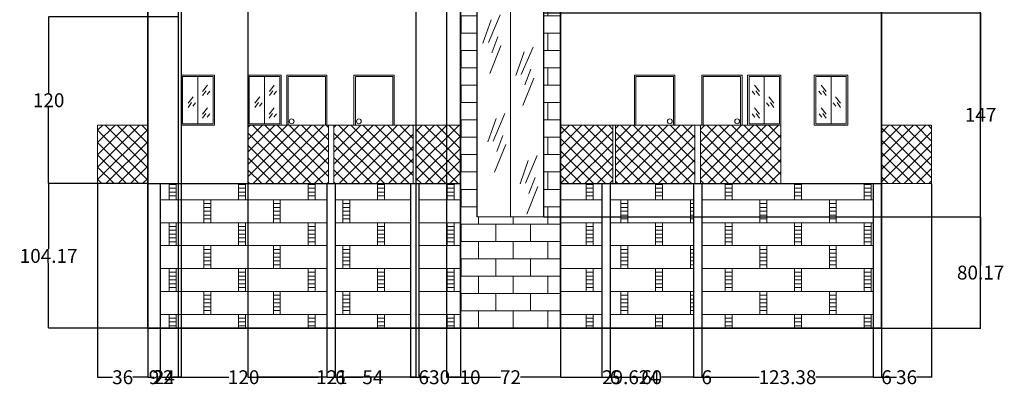
# Model space of a CAD drawing. Units: inches. Extents: x 183 to 891, y 196 to 984.
# Tile 1 of 3: x 183 to 891, y 196 to 460. Entities that reach past the tile are written whole.
import ezdxf

# ---------------------------------------------------------------- set-up
doc = ezdxf.new("R2010")
doc.units = ezdxf.units.IN
doc.header["$MEASUREMENT"] = 0
for name, color, linetype, lineweight in [('A-ANNO-DIMS', 2, 'Continuous', 18), ('A-COLS', 1, 'Continuous', 30), ('A-DOOR', 3, 'Continuous', 20), ('A-FLOR', 7, 'Continuous', 30), ('A-GLAZ', 4, 'Continuous', 18), ('A-GLAZ-DETL', 4, 'Continuous', 13), ('A-RAIL', 7, 'Continuous', 20), ('A-RAIL-PATT', 8, 'Continuous', 13), ('A-WALL', 7, 'Continuous', 35), ('A-WALL-PATT', 251, 'Continuous', 13)]:
    doc.layers.add(name, color=color, linetype=linetype, lineweight=lineweight)
doc.styles.get("Standard").update_dxf_attribs({"font": 'arial.ttf'})
doc.dimstyles.get("Standard").update_dxf_attribs({"dimtxt": 10, "dimasz": 0.18, "dimexe": 0.18, "dimexo": 0.0625, "dimgap": 0.09, "dimtad": 0, "dimtih": 1, "dimtoh": 1, "dimdec": 0, "dimzin": 0, "dimdsep": 46, "dimlunit": 3, "dimtxsty": 'Standard', "dimcen": 0.09, "dimadec": 0, "dimazin": 0, "dimtfac": 1, "dimtdec": 0, "dimtofl": 0, "dimtmove": 0, "dimatfit": 3, "dimfxl": 1, "dimtolj": 1, "dimtzin": 0, "dimarcsym": 0})

# ---------------------------------------------------------------- blocks, each defined once
blk = doc.blocks.new('WIN-SASH-PAIR-22X34')
for p, q in [((11, 34), (11, 0)), ((18.11, 27.96), (14.53, 23.4)), ((16.98, 23.73), (14.53, 20.31)), ((19.74, 23.56), (17.79, 21.12)), ((7.74, 19.54), (4.16, 14.99)), ((6.61, 15.31), (4.16, 11.9)), ((9.37, 15.15), (7.42, 12.71)), ((18.01, 11.64), (14.43, 7.09)), ((16.87, 7.41), (14.43, 4)), ((19.64, 7.25), (17.69, 4.81))]:
    blk.add_line(p, q)
blk.add_lwpolyline([(0, 0), (22, 0), (22, 34), (0, 34)], close=True)
blk = doc.blocks.new('DOOR-BALCONY-ELEV-29')
for p, q in [((0, 0), (0, 36)), ((0, 36), (29, 36)), ((29, 36), (29, 0)), ((1, 35), (28, 35)), ((1, 0), (1, 35)), ((28, 35), (28, 0))]:
    blk.add_line(p, q)
blk.add_circle((3.53, 2.84), 1.74)
blk = doc.blocks.new('GLASS-REFLECTION-ELEV')
for p, q in [((5.95, 38.63), (0, 21.79)), ((12.39, 42.09), (3.96, 22.28)), ((10.9, 26.25), (6.44, 14.86)), ((12.89, 19.81), (4.96, 0))]:
    blk.add_line(p, q)
blk = doc.blocks.new('*D9')
at = {"layer": 'A-ANNO-DIMS', "color": 0, "lineweight": -2, "transparency": 16777216}
for p, q in [((571.66, 941.68), (874.04, 941.68)), ((873.86, 941.5), (873.86, 594.79)), ((873.86, 237.69), (873.86, 584.4)), ((802.66, 237.51), (874.04, 237.51))]:
    blk.add_line(p, q, dxfattribs=at)
at = {"layer": 'A-ANNO-DIMS', "color": 0, "transparency": 16777216}
for points in [[(873.83, 941.5), (873.89, 941.5), (873.86, 941.68)], [(873.83, 237.69), (873.89, 237.69), (873.86, 237.51)]]:
    blk.add_solid(points, dxfattribs=at)
at = {"layer": 'Defpoints', "color": 0, "transparency": 16777216}
for p in [(571.6, 941.68), (873.86, 941.68), (802.6, 237.51)]:
    blk.add_point(p, dxfattribs=at)
at = {"layer": 'A-ANNO-DIMS', "color": 0, "transparency": 16777216, "insert": (873.86, 589.59), "char_height": 10, "attachment_point": 5}
blk.add_mtext('\\A1;704.2', dxfattribs=at)
blk = doc.blocks.new('*D11')
at = {"layer": 'A-ANNO-DIMS', "color": 0, "lineweight": -2, "transparency": 16777216}
for p, q in [((238.6, 341.61), (238.6, 202.06)), ((274.6, 237.45), (274.6, 202.06)), ((238.78, 202.24), (249.35, 202.24)), ((274.42, 202.24), (263.84, 202.24))]:
    blk.add_line(p, q, dxfattribs=at)
at = {"layer": 'A-ANNO-DIMS', "color": 0, "transparency": 16777216}
for points in [[(238.78, 202.27), (238.78, 202.21), (238.6, 202.24)], [(274.42, 202.27), (274.42, 202.21), (274.6, 202.24)]]:
    blk.add_solid(points, dxfattribs=at)
at = {"layer": 'Defpoints', "color": 0, "transparency": 16777216}
for p in [(238.6, 341.68), (274.6, 237.51), (274.6, 202.24)]:
    blk.add_point(p, dxfattribs=at)
at = {"layer": 'A-ANNO-DIMS', "color": 0, "transparency": 16777216, "insert": (256.6, 202.24), "char_height": 10, "attachment_point": 5}
blk.add_mtext('\\A1;36', dxfattribs=at)
blk = doc.blocks.new('*D12')
at = {"layer": 'A-ANNO-DIMS', "color": 0, "lineweight": -2, "transparency": 16777216}
for p, q in [((274.6, 237.45), (274.6, 202.06)), ((283.6, 237.45), (283.6, 202.06)), ((274.78, 202.24), (275.72, 202.24)), ((283.42, 202.24), (282.48, 202.24))]:
    blk.add_line(p, q, dxfattribs=at)
at = {"layer": 'A-ANNO-DIMS', "color": 0, "transparency": 16777216}
for points in [[(274.78, 202.27), (274.78, 202.21), (274.6, 202.24)], [(283.42, 202.27), (283.42, 202.21), (283.6, 202.24)]]:
    blk.add_solid(points, dxfattribs=at)
at = {"layer": 'Defpoints', "color": 0, "transparency": 16777216}
for p in [(274.6, 237.51), (283.6, 237.51), (283.6, 202.24)]:
    blk.add_point(p, dxfattribs=at)
at = {"layer": 'A-ANNO-DIMS', "color": 0, "transparency": 16777216, "insert": (279.1, 202.24), "char_height": 10, "attachment_point": 5}
blk.add_mtext('\\A1;9', dxfattribs=at)
blk = doc.blocks.new('*D13')
at = {"layer": 'A-ANNO-DIMS', "color": 0, "lineweight": -2, "transparency": 16777216}
for p, q in [((283.6, 237.45), (283.6, 202.06)), ((403.6, 237.45), (403.6, 202.06)), ((283.78, 202.24), (332.95, 202.24)), ((403.42, 202.24), (354.25, 202.24))]:
    blk.add_line(p, q, dxfattribs=at)
at = {"layer": 'A-ANNO-DIMS', "color": 0, "transparency": 16777216}
for points in [[(283.78, 202.27), (283.78, 202.21), (283.6, 202.24)], [(403.42, 202.27), (403.42, 202.21), (403.6, 202.24)]]:
    blk.add_solid(points, dxfattribs=at)
at = {"layer": 'Defpoints', "color": 0, "transparency": 16777216}
for p in [(283.6, 237.51), (403.6, 237.51), (403.6, 202.24)]:
    blk.add_point(p, dxfattribs=at)
at = {"layer": 'A-ANNO-DIMS', "color": 0, "transparency": 16777216, "insert": (343.6, 202.24), "char_height": 10, "attachment_point": 5}
blk.add_mtext('\\A1;120', dxfattribs=at)
blk = doc.blocks.new('*D14')
at = {"layer": 'A-ANNO-DIMS', "color": 0, "lineweight": -2, "transparency": 16777216}
for p, q in [((403.6, 237.45), (403.6, 202.06)), ((409.6, 237.45), (409.6, 202.06)), ((403.78, 202.24), (409.42, 202.24)), ((409.6, 202.24), (409.78, 202.24))]:
    blk.add_line(p, q, dxfattribs=at)
at = {"layer": 'A-ANNO-DIMS', "color": 0, "transparency": 16777216}
for points in [[(403.78, 202.27), (403.78, 202.21), (403.6, 202.24)], [(409.42, 202.27), (409.42, 202.21), (409.6, 202.24)]]:
    blk.add_solid(points, dxfattribs=at)
at = {"layer": 'Defpoints', "color": 0, "transparency": 16777216}
for p in [(403.6, 237.51), (409.6, 237.51), (409.6, 202.24)]:
    blk.add_point(p, dxfattribs=at)
at = {"layer": 'A-ANNO-DIMS', "color": 0, "transparency": 16777216, "insert": (413.17, 202.24), "char_height": 10, "attachment_point": 5}
blk.add_mtext('\\A1;6', dxfattribs=at)
blk = doc.blocks.new('*D15')
at = {"layer": 'A-ANNO-DIMS', "color": 0, "lineweight": -2, "transparency": 16777216}
for p, q in [((409.6, 237.45), (409.6, 202.06)), ((463.6, 237.45), (463.6, 202.06)), ((409.78, 202.24), (429.37, 202.24)), ((463.42, 202.24), (443.83, 202.24))]:
    blk.add_line(p, q, dxfattribs=at)
at = {"layer": 'A-ANNO-DIMS', "color": 0, "transparency": 16777216}
for points in [[(409.78, 202.27), (409.78, 202.21), (409.6, 202.24)], [(463.42, 202.27), (463.42, 202.21), (463.6, 202.24)]]:
    blk.add_solid(points, dxfattribs=at)
at = {"layer": 'Defpoints', "color": 0, "transparency": 16777216}
for p in [(409.6, 237.51), (463.6, 237.51), (463.6, 202.24)]:
    blk.add_point(p, dxfattribs=at)
at = {"layer": 'A-ANNO-DIMS', "color": 0, "transparency": 16777216, "insert": (436.6, 202.24), "char_height": 10, "attachment_point": 5}
blk.add_mtext('\\A1;54', dxfattribs=at)
blk = doc.blocks.new('*D16')
at = {"layer": 'A-ANNO-DIMS', "color": 0, "lineweight": -2, "transparency": 16777216}
for p, q in [((463.6, 237.45), (463.6, 202.06)), ((469.6, 237.45), (469.6, 202.06)), ((463.78, 202.24), (469.42, 202.24)), ((469.6, 202.24), (469.78, 202.24))]:
    blk.add_line(p, q, dxfattribs=at)
at = {"layer": 'A-ANNO-DIMS', "color": 0, "transparency": 16777216}
for points in [[(463.78, 202.27), (463.78, 202.21), (463.6, 202.24)], [(469.42, 202.27), (469.42, 202.21), (469.6, 202.24)]]:
    blk.add_solid(points, dxfattribs=at)
at = {"layer": 'Defpoints', "color": 0, "transparency": 16777216}
for p in [(463.6, 237.51), (469.6, 237.51), (469.6, 202.24)]:
    blk.add_point(p, dxfattribs=at)
at = {"layer": 'A-ANNO-DIMS', "color": 0, "transparency": 16777216, "insert": (473.17, 202.24), "char_height": 10, "attachment_point": 5}
blk.add_mtext('\\A1;6', dxfattribs=at)
blk = doc.blocks.new('*D17')
at = {"layer": 'A-ANNO-DIMS', "color": 0, "lineweight": -2, "transparency": 16777216}
for p, q in [((469.6, 237.45), (469.6, 202.06)), ((499.6, 237.45), (499.6, 202.06)), ((469.78, 202.24), (477.37, 202.24)), ((499.42, 202.24), (491.83, 202.24))]:
    blk.add_line(p, q, dxfattribs=at)
at = {"layer": 'A-ANNO-DIMS', "color": 0, "transparency": 16777216}
for points in [[(469.78, 202.27), (469.78, 202.21), (469.6, 202.24)], [(499.42, 202.27), (499.42, 202.21), (499.6, 202.24)]]:
    blk.add_solid(points, dxfattribs=at)
at = {"layer": 'Defpoints', "color": 0, "transparency": 16777216}
for p in [(469.6, 237.51), (499.6, 237.51), (499.6, 202.24)]:
    blk.add_point(p, dxfattribs=at)
at = {"layer": 'A-ANNO-DIMS', "color": 0, "transparency": 16777216, "insert": (484.6, 202.24), "char_height": 10, "attachment_point": 5}
blk.add_mtext('\\A1;30', dxfattribs=at)
blk = doc.blocks.new('*D18')
at = {"layer": 'A-ANNO-DIMS', "color": 0, "lineweight": -2, "transparency": 16777216}
for p, q in [((499.6, 237.45), (499.6, 202.06)), ((571.6, 237.45), (571.6, 202.06)), ((499.78, 202.24), (528.44, 202.24)), ((571.42, 202.24), (542.76, 202.24))]:
    blk.add_line(p, q, dxfattribs=at)
at = {"layer": 'A-ANNO-DIMS', "color": 0, "transparency": 16777216}
for points in [[(499.78, 202.27), (499.78, 202.21), (499.6, 202.24)], [(571.42, 202.27), (571.42, 202.21), (571.6, 202.24)]]:
    blk.add_solid(points, dxfattribs=at)
at = {"layer": 'Defpoints', "color": 0, "transparency": 16777216}
for p in [(499.6, 237.51), (571.6, 237.51), (571.6, 202.24)]:
    blk.add_point(p, dxfattribs=at)
at = {"layer": 'A-ANNO-DIMS', "color": 0, "transparency": 16777216, "insert": (535.6, 202.24), "char_height": 10, "attachment_point": 5}
blk.add_mtext('\\A1;72', dxfattribs=at)
blk = doc.blocks.new('*D19')
at = {"layer": 'A-ANNO-DIMS', "color": 0, "lineweight": -2, "transparency": 16777216}
for p, q in [((571.6, 237.45), (571.6, 202.06)), ((601.22, 237.45), (601.22, 202.06)), ((571.78, 202.24), (601.04, 202.24)), ((601.22, 202.24), (601.4, 202.24))]:
    blk.add_line(p, q, dxfattribs=at)
at = {"layer": 'A-ANNO-DIMS', "color": 0, "transparency": 16777216}
for points in [[(571.78, 202.27), (571.78, 202.21), (571.6, 202.24)], [(601.04, 202.27), (601.04, 202.21), (601.22, 202.24)]]:
    blk.add_solid(points, dxfattribs=at)
at = {"layer": 'Defpoints', "color": 0, "transparency": 16777216}
for p in [(571.6, 237.51), (601.22, 237.51), (601.22, 202.24)]:
    blk.add_point(p, dxfattribs=at)
at = {"layer": 'A-ANNO-DIMS', "color": 0, "transparency": 16777216, "insert": (622.31, 202.24), "char_height": 10, "attachment_point": 5}
blk.add_mtext('\\A1;29.624', dxfattribs=at)
blk = doc.blocks.new('*D20')
at = {"layer": 'A-ANNO-DIMS', "color": 0, "lineweight": -2, "transparency": 16777216}
for p, q in [((601.22, 237.45), (601.22, 202.06)), ((607.22, 237.45), (607.22, 202.06)), ((601.4, 202.24), (607.04, 202.24)), ((607.22, 202.24), (607.4, 202.24))]:
    blk.add_line(p, q, dxfattribs=at)
at = {"layer": 'A-ANNO-DIMS', "color": 0, "transparency": 16777216}
for points in [[(601.4, 202.27), (601.4, 202.21), (601.22, 202.24)], [(607.04, 202.27), (607.04, 202.21), (607.22, 202.24)]]:
    blk.add_solid(points, dxfattribs=at)
at = {"layer": 'Defpoints', "color": 0, "transparency": 16777216}
for p in [(601.22, 237.51), (607.22, 237.51), (607.22, 202.24)]:
    blk.add_point(p, dxfattribs=at)
at = {"layer": 'A-ANNO-DIMS', "color": 0, "transparency": 16777216, "insert": (610.79, 202.24), "char_height": 10, "attachment_point": 5}
blk.add_mtext('\\A1;6', dxfattribs=at)
blk = doc.blocks.new('*D21')
at = {"layer": 'A-ANNO-DIMS', "color": 0, "lineweight": -2, "transparency": 16777216}
for p, q in [((607.22, 237.45), (607.22, 202.06)), ((667.22, 237.45), (667.22, 202.06)), ((607.4, 202.24), (629.96, 202.24)), ((667.04, 202.24), (644.49, 202.24))]:
    blk.add_line(p, q, dxfattribs=at)
at = {"layer": 'A-ANNO-DIMS', "color": 0, "transparency": 16777216}
for points in [[(607.4, 202.27), (607.4, 202.21), (607.22, 202.24)], [(667.04, 202.27), (667.04, 202.21), (667.22, 202.24)]]:
    blk.add_solid(points, dxfattribs=at)
at = {"layer": 'Defpoints', "color": 0, "transparency": 16777216}
for p in [(607.22, 237.51), (667.22, 237.51), (667.22, 202.24)]:
    blk.add_point(p, dxfattribs=at)
at = {"layer": 'A-ANNO-DIMS', "color": 0, "transparency": 16777216, "insert": (637.22, 202.24), "char_height": 10, "attachment_point": 5}
blk.add_mtext('\\A1;60', dxfattribs=at)
blk = doc.blocks.new('*D22')
at = {"layer": 'A-ANNO-DIMS', "color": 0, "lineweight": -2, "transparency": 16777216}
for p, q in [((667.22, 237.45), (667.22, 202.06)), ((673.22, 237.45), (673.22, 202.06)), ((667.4, 202.24), (673.04, 202.24)), ((673.22, 202.24), (673.4, 202.24))]:
    blk.add_line(p, q, dxfattribs=at)
at = {"layer": 'A-ANNO-DIMS', "color": 0, "transparency": 16777216}
for points in [[(667.4, 202.27), (667.4, 202.21), (667.22, 202.24)], [(673.04, 202.27), (673.04, 202.21), (673.22, 202.24)]]:
    blk.add_solid(points, dxfattribs=at)
at = {"layer": 'Defpoints', "color": 0, "transparency": 16777216}
for p in [(667.22, 237.51), (673.22, 237.51), (673.22, 202.24)]:
    blk.add_point(p, dxfattribs=at)
at = {"layer": 'A-ANNO-DIMS', "color": 0, "transparency": 16777216, "insert": (676.79, 202.24), "char_height": 10, "attachment_point": 5}
blk.add_mtext('\\A1;6', dxfattribs=at)
blk = doc.blocks.new('*D23')
at = {"layer": 'A-ANNO-DIMS', "color": 0, "lineweight": -2, "transparency": 16777216}
for p, q in [((673.22, 237.45), (673.22, 202.06)), ((796.6, 237.45), (796.6, 202.06)), ((673.4, 202.24), (714.52, 202.24)), ((796.42, 202.24), (755.3, 202.24))]:
    blk.add_line(p, q, dxfattribs=at)
at = {"layer": 'A-ANNO-DIMS', "color": 0, "transparency": 16777216}
for points in [[(673.4, 202.27), (673.4, 202.21), (673.22, 202.24)], [(796.42, 202.27), (796.42, 202.21), (796.6, 202.24)]]:
    blk.add_solid(points, dxfattribs=at)
at = {"layer": 'Defpoints', "color": 0, "transparency": 16777216}
for p in [(673.22, 237.51), (796.6, 237.51), (796.6, 202.24)]:
    blk.add_point(p, dxfattribs=at)
at = {"layer": 'A-ANNO-DIMS', "color": 0, "transparency": 16777216, "insert": (734.91, 202.24), "char_height": 10, "attachment_point": 5}
blk.add_mtext('\\A1;123.38', dxfattribs=at)
blk = doc.blocks.new('*D24')
at = {"layer": 'A-ANNO-DIMS', "color": 0, "lineweight": -2, "transparency": 16777216}
for p, q in [((796.6, 237.45), (796.6, 202.06)), ((802.6, 237.45), (802.6, 202.06)), ((796.78, 202.24), (802.42, 202.24)), ((802.6, 202.24), (802.78, 202.24))]:
    blk.add_line(p, q, dxfattribs=at)
at = {"layer": 'A-ANNO-DIMS', "color": 0, "transparency": 16777216}
for points in [[(796.78, 202.27), (796.78, 202.21), (796.6, 202.24)], [(802.42, 202.27), (802.42, 202.21), (802.6, 202.24)]]:
    blk.add_solid(points, dxfattribs=at)
at = {"layer": 'Defpoints', "color": 0, "transparency": 16777216}
for p in [(796.6, 237.51), (802.6, 237.51), (802.6, 202.24)]:
    blk.add_point(p, dxfattribs=at)
at = {"layer": 'A-ANNO-DIMS', "color": 0, "transparency": 16777216, "insert": (806.17, 202.24), "char_height": 10, "attachment_point": 5}
blk.add_mtext('\\A1;6', dxfattribs=at)
blk = doc.blocks.new('*D25')
at = {"layer": 'A-ANNO-DIMS', "color": 0, "lineweight": -2, "transparency": 16777216}
for p, q in [((838.6, 341.61), (838.6, 202.06)), ((802.6, 237.45), (802.6, 202.06)), ((802.78, 202.24), (813.35, 202.24)), ((838.42, 202.24), (827.84, 202.24))]:
    blk.add_line(p, q, dxfattribs=at)
at = {"layer": 'A-ANNO-DIMS', "color": 0, "transparency": 16777216}
for points in [[(802.78, 202.27), (802.78, 202.21), (802.6, 202.24)], [(838.42, 202.27), (838.42, 202.21), (838.6, 202.24)]]:
    blk.add_solid(points, dxfattribs=at)
at = {"layer": 'Defpoints', "color": 0, "transparency": 16777216}
for p in [(838.6, 341.68), (802.6, 237.51), (838.6, 202.24)]:
    blk.add_point(p, dxfattribs=at)
at = {"layer": 'A-ANNO-DIMS', "color": 0, "transparency": 16777216, "insert": (820.6, 202.24), "char_height": 10, "attachment_point": 5}
blk.add_mtext('\\A1;36', dxfattribs=at)
blk = doc.blocks.new('*D26')
at = {"layer": 'A-ANNO-DIMS', "color": 0, "lineweight": -2, "transparency": 16777216}
for p, q in [((274.54, 341.68), (203.15, 341.68)), ((203.33, 341.5), (203.33, 294.79)), ((203.33, 237.69), (203.33, 284.4)), ((274.54, 237.51), (203.15, 237.51))]:
    blk.add_line(p, q, dxfattribs=at)
at = {"layer": 'A-ANNO-DIMS', "color": 0, "transparency": 16777216}
for points in [[(203.3, 341.5), (203.36, 341.5), (203.33, 341.68)], [(203.3, 237.69), (203.36, 237.69), (203.33, 237.51)]]:
    blk.add_solid(points, dxfattribs=at)
at = {"layer": 'Defpoints', "color": 0, "transparency": 16777216}
for p in [(203.33, 341.68), (274.6, 341.68), (274.6, 237.51)]:
    blk.add_point(p, dxfattribs=at)
at = {"layer": 'A-ANNO-DIMS', "color": 0, "transparency": 16777216, "insert": (203.33, 289.59), "char_height": 10, "attachment_point": 5}
blk.add_mtext('\\A1;104.17', dxfattribs=at)
blk = doc.blocks.new('*D27')
at = {"layer": 'A-ANNO-DIMS', "color": 0, "lineweight": -2, "transparency": 16777216}
for p, q in [((296.54, 461.68), (203.15, 461.68)), ((203.33, 461.5), (203.33, 406.87)), ((203.33, 341.86), (203.33, 396.48)), ((274.54, 341.68), (203.15, 341.68))]:
    blk.add_line(p, q, dxfattribs=at)
at = {"layer": 'A-ANNO-DIMS', "color": 0, "transparency": 16777216}
for points in [[(203.3, 461.5), (203.36, 461.5), (203.33, 461.68)], [(203.3, 341.86), (203.36, 341.86), (203.33, 341.68)]]:
    blk.add_solid(points, dxfattribs=at)
at = {"layer": 'Defpoints', "color": 0, "transparency": 16777216}
for p in [(203.33, 461.68), (296.6, 461.68), (274.6, 341.68)]:
    blk.add_point(p, dxfattribs=at)
at = {"layer": 'A-ANNO-DIMS', "color": 0, "transparency": 16777216, "insert": (203.33, 401.68), "char_height": 10, "attachment_point": 5}
blk.add_mtext('\\A1;120', dxfattribs=at)
blk = doc.blocks.new('*D36')
at = {"layer": 'A-ANNO-DIMS', "color": 0, "lineweight": -2, "transparency": 16777216}
for p, q in [((499.6, 237.57), (499.6, 977.12)), ((499.78, 976.94), (511.42, 976.94)), ((511.6, 317.74), (511.6, 977.12)), ((511.6, 976.94), (511.78, 976.94))]:
    blk.add_line(p, q, dxfattribs=at)
at = {"layer": 'A-ANNO-DIMS', "color": 0, "transparency": 16777216}
for points in [[(499.78, 976.97), (499.78, 976.91), (499.6, 976.94)], [(511.42, 976.97), (511.42, 976.91), (511.6, 976.94)]]:
    blk.add_solid(points, dxfattribs=at)
at = {"layer": 'Defpoints', "color": 0, "transparency": 16777216}
for p in [(511.6, 976.94), (511.6, 317.68), (499.6, 237.51)]:
    blk.add_point(p, dxfattribs=at)
at = {"layer": 'A-ANNO-DIMS', "color": 0, "transparency": 16777216, "insert": (518.51, 976.94), "char_height": 10, "attachment_point": 5}
blk.add_mtext('\\A1;12', dxfattribs=at)
blk = doc.blocks.new('*D37')
at = {"layer": 'A-ANNO-DIMS', "color": 0, "lineweight": -2, "transparency": 16777216}
for p, q in [((559.6, 317.74), (559.6, 977.12)), ((559.78, 976.94), (571.42, 976.94)), ((571.6, 237.57), (571.6, 977.12)), ((571.6, 976.94), (571.78, 976.94))]:
    blk.add_line(p, q, dxfattribs=at)
at = {"layer": 'A-ANNO-DIMS', "color": 0, "transparency": 16777216}
for points in [[(559.78, 976.97), (559.78, 976.91), (559.6, 976.94)], [(571.42, 976.97), (571.42, 976.91), (571.6, 976.94)]]:
    blk.add_solid(points, dxfattribs=at)
at = {"layer": 'Defpoints', "color": 0, "transparency": 16777216}
for p in [(571.6, 976.94), (559.6, 317.68), (571.6, 237.51)]:
    blk.add_point(p, dxfattribs=at)
at = {"layer": 'A-ANNO-DIMS', "color": 0, "transparency": 16777216, "insert": (578.51, 976.94), "char_height": 10, "attachment_point": 5}
blk.add_mtext('\\A1;12', dxfattribs=at)
blk = doc.blocks.new('*D38')
at = {"layer": 'A-ANNO-DIMS', "color": 0, "lineweight": -2, "transparency": 16777216}
for p, q in [((559.66, 317.68), (874.04, 317.68)), ((873.86, 317.5), (873.86, 282.79)), ((873.86, 237.69), (873.86, 272.4)), ((571.66, 237.51), (874.04, 237.51))]:
    blk.add_line(p, q, dxfattribs=at)
at = {"layer": 'A-ANNO-DIMS', "color": 0, "transparency": 16777216}
for points in [[(873.83, 317.5), (873.89, 317.5), (873.86, 317.68)], [(873.83, 237.69), (873.89, 237.69), (873.86, 237.51)]]:
    blk.add_solid(points, dxfattribs=at)
at = {"layer": 'Defpoints', "color": 0, "transparency": 16777216}
for p in [(559.6, 317.68), (571.6, 237.51), (873.86, 237.51)]:
    blk.add_point(p, dxfattribs=at)
at = {"layer": 'A-ANNO-DIMS', "color": 0, "transparency": 16777216, "insert": (873.86, 277.59), "char_height": 10, "attachment_point": 5}
blk.add_mtext('\\A1;80.17', dxfattribs=at)
blk = doc.blocks.new('*D39')
at = {"layer": 'A-ANNO-DIMS', "color": 0, "lineweight": -2, "transparency": 16777216}
for p, q in [((559.66, 464.68), (874.04, 464.68)), ((873.86, 464.5), (873.86, 396.29)), ((873.86, 317.86), (873.86, 386.06)), ((559.66, 317.68), (874.04, 317.68))]:
    blk.add_line(p, q, dxfattribs=at)
at = {"layer": 'A-ANNO-DIMS', "color": 0, "transparency": 16777216}
for points in [[(873.83, 464.5), (873.89, 464.5), (873.86, 464.68)], [(873.83, 317.86), (873.89, 317.86), (873.86, 317.68)]]:
    blk.add_solid(points, dxfattribs=at)
at = {"layer": 'Defpoints', "color": 0, "transparency": 16777216}
for p in [(559.6, 464.68), (873.86, 464.68), (559.6, 317.68)]:
    blk.add_point(p, dxfattribs=at)
at = {"layer": 'A-ANNO-DIMS', "color": 0, "transparency": 16777216, "insert": (873.86, 391.18), "char_height": 10, "attachment_point": 5}
blk.add_mtext('\\A1;147', dxfattribs=at)
blk = doc.blocks.new('*D40')
at = {"layer": 'A-ANNO-DIMS', "color": 0, "lineweight": -2, "transparency": 16777216}
for p, q in [((274.6, 742.8), (274.6, 202.06)), ((298.6, 743.61), (298.6, 202.06)), ((274.78, 202.24), (279.28, 202.24)), ((298.42, 202.24), (293.92, 202.24))]:
    blk.add_line(p, q, dxfattribs=at)
at = {"layer": 'A-ANNO-DIMS', "color": 0, "transparency": 16777216}
for points in [[(274.78, 202.27), (274.78, 202.21), (274.6, 202.24)], [(298.42, 202.27), (298.42, 202.21), (298.6, 202.24)]]:
    blk.add_solid(points, dxfattribs=at)
at = {"layer": 'Defpoints', "color": 0, "transparency": 16777216}
for p in [(274.6, 742.86), (298.6, 743.68), (298.6, 202.24)]:
    blk.add_point(p, dxfattribs=at)
at = {"layer": 'A-ANNO-DIMS', "color": 0, "transparency": 16777216, "insert": (286.6, 202.24), "char_height": 10, "attachment_point": 5}
blk.add_mtext('\\A1;24', dxfattribs=at)
blk = doc.blocks.new('*D44')
at = {"layer": 'A-ANNO-DIMS', "color": 0, "lineweight": -2, "transparency": 16777216}
for p, q in [((346.6, 701.61), (346.6, 202.06)), ((467.6, 701.61), (467.6, 202.06)), ((346.78, 202.24), (397.4, 202.24)), ((467.42, 202.24), (416.8, 202.24))]:
    blk.add_line(p, q, dxfattribs=at)
at = {"layer": 'A-ANNO-DIMS', "color": 0, "transparency": 16777216}
for points in [[(346.78, 202.27), (346.78, 202.21), (346.6, 202.24)], [(467.42, 202.27), (467.42, 202.21), (467.6, 202.24)]]:
    blk.add_solid(points, dxfattribs=at)
at = {"layer": 'Defpoints', "color": 0, "transparency": 16777216}
for p in [(346.6, 701.68), (467.6, 701.68), (467.6, 202.24)]:
    blk.add_point(p, dxfattribs=at)
at = {"layer": 'A-ANNO-DIMS', "color": 0, "transparency": 16777216, "insert": (407.1, 202.24), "char_height": 10, "attachment_point": 5}
blk.add_mtext('\\A1;121', dxfattribs=at)
blk = doc.blocks.new('*D46')
at = {"layer": 'A-ANNO-DIMS', "color": 0, "lineweight": -2, "transparency": 16777216}
for p, q in [((274.6, 821.61), (274.6, 202.06)), ((296.6, 811.61), (296.6, 202.06)), ((274.78, 202.24), (278.31, 202.24)), ((296.42, 202.24), (292.89, 202.24))]:
    blk.add_line(p, q, dxfattribs=at)
at = {"layer": 'A-ANNO-DIMS', "color": 0, "transparency": 16777216}
for points in [[(274.78, 202.27), (274.78, 202.21), (274.6, 202.24)], [(296.42, 202.27), (296.42, 202.21), (296.6, 202.24)]]:
    blk.add_solid(points, dxfattribs=at)
at = {"layer": 'Defpoints', "color": 0, "transparency": 16777216}
for p in [(274.6, 821.68), (296.6, 811.68), (296.6, 202.24)]:
    blk.add_point(p, dxfattribs=at)
at = {"layer": 'A-ANNO-DIMS', "color": 0, "transparency": 16777216, "insert": (285.6, 202.24), "char_height": 10, "attachment_point": 5}
blk.add_mtext('\\A1;22', dxfattribs=at)
blk = doc.blocks.new('*D47')
at = {"layer": 'A-ANNO-DIMS', "color": 0, "lineweight": -2, "transparency": 16777216}
for p, q in [((499.6, 821.61), (499.6, 202.06)), ((489.6, 811.61), (489.6, 202.06)), ((489.78, 202.24), (499.42, 202.24)), ((499.6, 202.24), (499.78, 202.24))]:
    blk.add_line(p, q, dxfattribs=at)
at = {"layer": 'A-ANNO-DIMS', "color": 0, "transparency": 16777216}
for points in [[(489.78, 202.27), (489.78, 202.21), (489.6, 202.24)], [(499.42, 202.27), (499.42, 202.21), (499.6, 202.24)]]:
    blk.add_solid(points, dxfattribs=at)
at = {"layer": 'Defpoints', "color": 0, "transparency": 16777216}
for p in [(499.6, 821.68), (489.6, 811.68), (499.6, 202.24)]:
    blk.add_point(p, dxfattribs=at)
at = {"layer": 'A-ANNO-DIMS', "color": 0, "transparency": 16777216, "insert": (506.54, 202.24), "char_height": 10, "attachment_point": 5}
blk.add_mtext('\\A1;10', dxfattribs=at)

msp = doc.modelspace()

# ---------------------------------------------------------------- hatches: boundary and pattern name
at = {"layer": 'A-RAIL-PATT'}
h = msp.add_hatch(dxfattribs=at)
h.set_pattern_fill('ANSI37', color=256, scale=50)
h.paths.add_polyline_path([(404.599, 743.6754), (346.599, 743.6754), (346.599, 701.6754), (404.599, 701.6754)])
h.paths.add_polyline_path([(465.599, 743.6754), (408.599, 743.6754), (408.599, 701.6754), (465.599, 701.6754)])
h.paths.add_polyline_path([(668.2227, 743.6754), (611.2227, 743.6754), (611.2227, 701.6754), (668.2227, 701.6754)])
h.paths.add_polyline_path([(730.2227, 743.6754), (706.2227, 743.6754), (672.2227, 743.6754), (672.2227, 701.6754), (730.2227, 701.6754)])
h.paths.add_polyline_path([(838.599, 743.6754), (802.599, 743.6754), (802.599, 701.6754), (838.599, 701.6754)])
h.paths.add_polyline_path([(274.599, 742.8641), (238.599, 742.8641), (238.599, 700.8641), (274.599, 700.8641)])
h.paths.add_polyline_path([(274.599, 625.2404), (238.599, 625.2404), (238.599, 583.2404), (274.599, 583.2404)])
h.paths.add_polyline_path([(404.599, 623.6754), (346.599, 623.6754), (346.599, 581.6754), (404.599, 581.6754)])
h.paths.add_polyline_path([(465.599, 623.6754), (408.599, 623.6754), (408.599, 581.6754), (465.599, 581.6754)])
h.paths.add_polyline_path([(668.2227, 623.6754), (611.2227, 623.6754), (611.2227, 581.6754), (668.2227, 581.6754)])
h.paths.add_polyline_path([(730.2227, 623.6754), (672.2227, 623.6754), (672.2227, 581.6754), (730.2227, 581.6754)])
h.paths.add_polyline_path([(838.599, 625.42), (802.599, 625.42), (802.599, 583.42), (838.599, 583.42)])
h.paths.add_polyline_path([(404.599, 515.6754), (346.599, 515.6754), (346.599, 473.6754), (404.599, 473.6754)])
h.paths.add_polyline_path([(465.599, 515.6754), (408.599, 515.6754), (408.599, 473.6754), (465.599, 473.6754)])
h.paths.add_polyline_path([(668.2227, 515.6754), (611.2227, 515.6754), (611.2227, 473.6754), (668.2227, 473.6754)])
h.paths.add_polyline_path([(730.2227, 515.6754), (706.2227, 515.6754), (672.2227, 515.6754), (672.2227, 473.6754), (730.2227, 473.6754)])
h.paths.add_polyline_path([(838.599, 514.8979), (802.599, 514.8979), (802.599, 472.8979), (838.599, 472.8979)])
h.paths.add_polyline_path([(668.2227, 383.6754), (611.2227, 383.6754), (611.2227, 341.6754), (668.2227, 341.6754)])
h.paths.add_polyline_path([(609.2227, 383.6754), (571.599, 383.6754), (571.599, 341.6754), (601.2227, 341.6754), (609.2227, 341.6754)])
h.paths.add_polyline_path([(730.2227, 383.6754), (672.2227, 383.6754), (672.2227, 341.6754), (730.2227, 341.6754)])
h.paths.add_polyline_path([(838.599, 383.6754), (802.599, 383.6754), (802.599, 341.6754), (838.599, 341.6754)])
h.paths.add_polyline_path([(499.599, 383.6754), (467.599, 383.6754), (467.599, 341.6754), (499.599, 341.6754)])
h.paths.add_polyline_path([(465.599, 383.6754), (408.599, 383.6754), (408.599, 341.6754), (465.599, 341.6754)])
h.paths.add_polyline_path([(404.599, 383.6754), (346.599, 383.6754), (346.599, 341.6754), (404.599, 341.6754)])
h.paths.add_polyline_path([(274.599, 383.6754), (238.599, 383.6754), (238.599, 341.6754), (274.599, 341.6754)])
h.paths.add_polyline_path([(274.599, 514.3451), (238.599, 514.3451), (238.599, 472.3451), (274.599, 472.3451)])
at = {"layer": 'A-WALL-PATT'}
h = msp.add_hatch(dxfattribs=at)
h.set_pattern_fill('BRICK', color=256, scale=50)
h.paths.add_polyline_path([(571.599, 341.6754), (571.599, 821.6754), (571.599, 905.6754), (571.599, 941.6754), (499.599, 941.6754), (499.599, 905.6754), (499.599, 821.6754), (499.599, 341.6754), (499.599, 237.5076), (571.599, 237.5076)])
h.paths.add_polyline_path([(511.599, 317.6754), (511.599, 905.6754), (559.599, 905.6754), (559.599, 317.6754)], flags=16)
h = msp.add_hatch(dxfattribs=at)
h.set_pattern_fill('BRSTONE', color=256, scale=50)
h.paths.add_polyline_path([(403.599, 341.6754), (283.599, 341.6754), (283.599, 237.5076), (403.599, 237.5076)])
h.paths.add_polyline_path([(463.599, 341.6754), (409.599, 341.6754), (409.599, 237.5076), (463.599, 237.5076)])
h.paths.add_polyline_path([(499.599, 341.6754), (469.599, 341.6754), (469.599, 237.5076), (499.599, 237.5076)])
h.paths.add_polyline_path([(601.2227, 341.6754), (571.599, 341.6754), (571.599, 237.5076), (601.2227, 237.5076)])
h.paths.add_polyline_path([(667.2227, 341.6754), (607.2227, 341.6754), (607.2227, 237.5076), (634.599, 237.5076), (667.2227, 237.5076)])
h.paths.add_polyline_path([(796.599, 341.6754), (673.2227, 341.6754), (673.2227, 237.5076), (796.599, 237.5076)])

# ---------------------------------------------------------------- linework, layer by layer
at = {"layer": 'A-COLS'}
for p, q in [((283.599, 341.6754), (283.599, 237.5076)), ((403.599, 341.6754), (403.599, 237.5076)), ((409.599, 341.6754), (409.599, 237.5076)), ((463.599, 341.6754), (463.599, 237.5076)), ((469.599, 341.6754), (469.599, 237.5076)), ((601.2227, 341.6754), (601.2227, 237.5076)), ((607.2227, 341.6754), (607.2227, 237.5076)), ((667.2227, 341.6754), (667.2227, 237.5076)), ((673.2227, 341.6754), (673.2227, 237.5076)), ((796.599, 341.6754), (796.599, 237.5076))]:
    msp.add_line(p, q, dxfattribs=at)
at = {"layer": 'A-FLOR'}
for p, q in [((274.599, 341.6754), (499.599, 341.6754)), ((571.599, 341.6754), (601.2227, 341.6754)), ((577.2227, 341.6754), (802.599, 341.6754))]:
    msp.add_line(p, q, dxfattribs=at)
at = {"layer": 'A-GLAZ'}
for p, q in [((535.599, 905.6754), (535.599, 317.6754)), ((535.599, 611.6754), (535.599, 317.6754)), ((298.599, 383.6754), (322.599, 383.6754)), ((772.599, 383.6754), (754.2227, 383.6754))]:
    msp.add_line(p, q, dxfattribs=at)
for points in [[(511.599, 905.6754), (559.599, 905.6754), (559.599, 317.6754), (511.599, 317.6754)], [(298.599, 383.6754), (322.599, 383.6754), (322.599, 419.6754), (298.599, 419.6754)], [(346.599, 383.6754), (370.599, 383.6754), (370.599, 419.6754), (346.599, 419.6754)], [(730.2227, 383.6754), (706.2227, 383.6754), (706.2227, 419.6754), (730.2227, 419.6754)], [(778.2227, 383.6754), (754.2227, 383.6754), (754.2227, 419.6754), (778.2227, 419.6754)]]:
    msp.add_lwpolyline(points, close=True, dxfattribs=at)
at = {"layer": 'A-RAIL'}
for p, q in [((238.599, 341.6754), (238.599, 383.6754)), ((238.599, 383.6754), (274.599, 383.6754)), ((346.599, 383.6754), (346.599, 341.6754)), ((346.599, 383.6754), (499.599, 383.6754)), ((370.599, 383.6754), (374.599, 383.6754)), ((404.599, 383.6754), (404.599, 341.8554)), ((408.599, 383.6754), (408.599, 341.8554)), ((465.599, 341.6754), (465.599, 383.6754)), ((467.599, 341.6754), (467.599, 383.6754)), ((730.2227, 383.6754), (571.599, 383.6754)), ((609.2227, 341.6754), (609.2227, 383.6754)), ((611.2227, 341.6754), (611.2227, 383.6754)), ((668.2227, 383.6754), (668.2227, 341.8554)), ((672.2227, 383.6754), (672.2227, 341.8554)), ((715.599, 383.6754), (711.599, 383.6754)), ((730.2227, 383.6754), (730.2227, 341.6754)), ((838.599, 383.6754), (802.599, 383.6754)), ((838.599, 341.6754), (838.599, 383.6754)), ((274.599, 341.6754), (238.599, 341.6754)), ((802.599, 341.6754), (838.599, 341.6754))]:
    msp.add_line(p, q, dxfattribs=at)
at = {"layer": 'A-WALL'}
for p, q in [((274.599, 863.6754), (274.599, 237.5076)), ((802.599, 237.5076), (802.599, 863.6754)), ((499.599, 821.6754), (499.599, 341.6754)), ((571.599, 821.6754), (571.599, 341.6754)), ((499.599, 341.6754), (499.599, 237.5076)), ((571.599, 237.5076), (571.599, 341.6754)), ((802.599, 341.6754), (802.599, 237.5076)), ((274.599, 237.5076), (634.599, 237.5076)), ((634.599, 237.5076), (796.599, 237.5076)), ((796.599, 237.5076), (802.599, 237.5076))]:
    msp.add_line(p, q, dxfattribs=at)

# ---------------------------------------------------------------- block references
at = {"layer": 'A-DOOR'}
for p in [(374.599, 383.675), (423.0255, 383.675)]:
    msp.add_blockref('DOOR-BALCONY-ELEV-29', p, dxfattribs=at)
at = {"layer": 'A-DOOR', "extrusion": (0, 0, -1), "zscale": -1}
for p in [(-653.7962, 383.675), (-702.2227, 383.675)]:
    msp.add_blockref('DOOR-BALCONY-ELEV-29', p, dxfattribs=at)
at = {"layer": 'A-GLAZ'}
for p in [(299.599, 384.675), (347.599, 384.675)]:
    msp.add_blockref('WIN-SASH-PAIR-22X34', p, dxfattribs=at)
at = {"layer": 'A-GLAZ', "extrusion": (0, 0, -1), "zscale": -1}
for p in [(-729.2227, 384.675), (-777.2227, 384.675)]:
    msp.add_blockref('WIN-SASH-PAIR-22X34', p, dxfattribs=at)
at = {"layer": 'A-GLAZ-DETL'}
for p in [(515.7286, 421.0131), (539.4389, 397.8267), (519.26, 349.9416), (542.4657, 319.6985)]:
    msp.add_blockref('GLASS-REFLECTION-ELEV', p, dxfattribs=at)

# ---------------------------------------------------------------- dimensions: what is measured, and where the dimension line sits
at = {"layer": 'A-ANNO-DIMS'}
for base, p1, p2, override, picture, middle in [((511.599, 976.9404), (499.599, 237.5076), (511.599, 317.6754), {"dimdec": 0, "dimlfac": 1, "dimrnd": 0, "dimzin": 0, "dimdsep": 46, "dimlunit": 2}, '*D36', (518.5095, 976.9404)), ((571.599, 976.9404), (559.599, 317.6754), (571.599, 237.5076), {"dimdec": 0, "dimlfac": 1, "dimrnd": 0, "dimzin": 0, "dimdsep": 46, "dimlunit": 2}, '*D37', (578.5095, 976.9404)), ((296.599, 202.2426), (274.599, 821.6754), (296.599, 811.6754), {"dimdec": 0, "dimlfac": 1, "dimrnd": 0, "dimzin": 0, "dimdsep": 46, "dimlunit": 2}, '*D46', (285.599, 202.2426)), ((499.599, 202.2426), (489.599, 811.6754), (499.599, 821.6754), {"dimdec": 0, "dimlfac": 1, "dimrnd": 0, "dimzin": 0, "dimdsep": 46, "dimlunit": 2}, '*D47', (506.5436, 202.2426)), ((298.599, 202.2426), (274.599, 742.8641), (298.599, 743.6754), {"dimdec": 0, "dimlfac": 1, "dimrnd": 0, "dimzin": 0, "dimdsep": 46, "dimlunit": 2}, '*D40', (286.599, 202.2426)), ((467.599, 202.2426), (346.599, 701.6754), (467.599, 701.6754), {"dimdec": 0, "dimlfac": 1, "dimrnd": 0, "dimzin": 0, "dimdsep": 46, "dimlunit": 2}, '*D44', (407.099, 202.2426)), ((274.599, 202.2426), (238.599, 341.6754), (274.599, 237.5076), {"dimdec": 0, "dimlfac": 1, "dimrnd": 0, "dimzin": 0, "dimdsep": 46, "dimlunit": 2}, '*D11', (256.599, 202.2426)), ((838.599, 202.2426), (802.599, 237.5076), (838.599, 341.6754), {"dimdec": 0, "dimlfac": 1, "dimrnd": 0, "dimzin": 0, "dimdsep": 46, "dimlunit": 2}, '*D25', (820.599, 202.2426)), ((283.599, 202.2426), (274.599, 237.5076), (283.599, 237.5076), {"dimdec": 0, "dimlfac": 1, "dimrnd": 0, "dimzin": 0, "dimdsep": 46, "dimlunit": 2}, '*D12', (279.099, 202.2426)), ((403.599, 202.2426), (283.599, 237.5076), (403.599, 237.5076), {"dimdec": 0, "dimlfac": 1, "dimrnd": 0, "dimzin": 0, "dimdsep": 46, "dimlunit": 2}, '*D13', (343.599, 202.2426)), ((409.599, 202.2426), (403.599, 237.5076), (409.599, 237.5076), {"dimdec": 0, "dimlfac": 1, "dimrnd": 0, "dimzin": 0, "dimdsep": 46, "dimlunit": 2}, '*D14', (413.1705, 202.2426)), ((463.599, 202.2426), (409.599, 237.5076), (463.599, 237.5076), {"dimdec": 0, "dimlfac": 1, "dimrnd": 0, "dimzin": 0, "dimdsep": 46, "dimlunit": 2}, '*D15', (436.599, 202.2426)), ((469.599, 202.2426), (463.599, 237.5076), (469.599, 237.5076), {"dimdec": 0, "dimlfac": 1, "dimrnd": 0, "dimzin": 0, "dimdsep": 46, "dimlunit": 2}, '*D16', (473.1705, 202.2426)), ((499.599, 202.2426), (469.599, 237.5076), (499.599, 237.5076), {"dimdec": 0, "dimlfac": 1, "dimrnd": 0, "dimzin": 0, "dimdsep": 46, "dimlunit": 2}, '*D17', (484.599, 202.2426)), ((571.599, 202.2426), (499.599, 237.5076), (571.599, 237.5076), {"dimdec": 0, "dimlfac": 1, "dimrnd": 0, "dimzin": 0, "dimdsep": 46, "dimlunit": 2}, '*D18', (535.599, 202.2426)), ((601.2227, 202.2426), (571.599, 237.5076), (601.2227, 237.5076), {"dimdec": 3, "dimlfac": 1, "dimrnd": 0, "dimzin": 0, "dimdsep": 46, "dimlunit": 2}, '*D19', (622.3147, 202.2426)), ((607.2227, 202.2426), (601.2227, 237.5076), (607.2227, 237.5076), {"dimdec": 0, "dimlfac": 1, "dimrnd": 0, "dimzin": 0, "dimdsep": 46, "dimlunit": 2}, '*D20', (610.7942, 202.2426)), ((667.2227, 202.2426), (607.2227, 237.5076), (667.2227, 237.5076), {"dimdec": 0, "dimlfac": 1, "dimrnd": 0, "dimzin": 0, "dimdsep": 46, "dimlunit": 2}, '*D21', (637.2227, 202.2426)), ((673.2227, 202.2426), (667.2227, 237.5076), (673.2227, 237.5076), {"dimdec": 0, "dimlfac": 1, "dimrnd": 0, "dimzin": 0, "dimdsep": 46, "dimlunit": 2}, '*D22', (676.7942, 202.2426)), ((796.599, 202.2426), (673.2227, 237.5076), (796.599, 237.5076), {"dimdec": 2, "dimlfac": 1, "dimrnd": 0, "dimzin": 0, "dimdsep": 46, "dimlunit": 2}, '*D23', (734.9109, 202.2426)), ((802.599, 202.2426), (796.599, 237.5076), (802.599, 237.5076), {"dimdec": 0, "dimlfac": 1, "dimrnd": 0, "dimzin": 0, "dimdsep": 46, "dimlunit": 2}, '*D24', (806.1705, 202.2426))]:
    dim = msp.add_linear_dim(base=base, p1=p1, p2=p2, dimstyle='Standard', override=override, dxfattribs=at)
    dim.commit()
    dim.dimension.update_dxf_attribs({"geometry": picture, "text_midpoint": middle})
for base, p1, p2, override, picture, middle in [((873.864, 941.6754), (802.599, 237.5076), (571.599, 941.6754), {"dimdec": 1, "dimlfac": 1, "dimrnd": 0, "dimzin": 0, "dimdsep": 46, "dimlunit": 2}, '*D9', (873.864, 589.5915)), ((203.334, 461.6754), (274.599, 341.6754), (296.599, 461.6754), {"dimdec": 0, "dimlfac": 1, "dimrnd": 0, "dimzin": 0, "dimdsep": 46, "dimlunit": 2}, '*D27', (203.334, 401.6754)), ((873.864, 464.6754), (559.599, 317.6754), (559.599, 464.6754), {"dimdec": 0, "dimlfac": 1, "dimrnd": 0, "dimzin": 0, "dimdsep": 46, "dimlunit": 2}, '*D39', (873.864, 391.1754)), ((203.334, 341.6754), (274.599, 237.5076), (274.599, 341.6754), {"dimdec": 2, "dimlfac": 1, "dimrnd": 0, "dimzin": 0, "dimdsep": 46, "dimlunit": 2}, '*D26', (203.334, 289.5915)), ((873.864, 237.5076), (559.599, 317.6754), (571.599, 237.5076), {"dimdec": 2, "dimlfac": 1, "dimrnd": 0, "dimzin": 0, "dimdsep": 46, "dimlunit": 2}, '*D38', (873.864, 277.5915))]:
    dim = msp.add_linear_dim(base=base, p1=p1, p2=p2, angle=90, dimstyle='Standard', override=override, dxfattribs=at)
    dim.commit()
    dim.dimension.update_dxf_attribs({"geometry": picture, "text_midpoint": middle})

doc.saveas('drawing.dxf')
